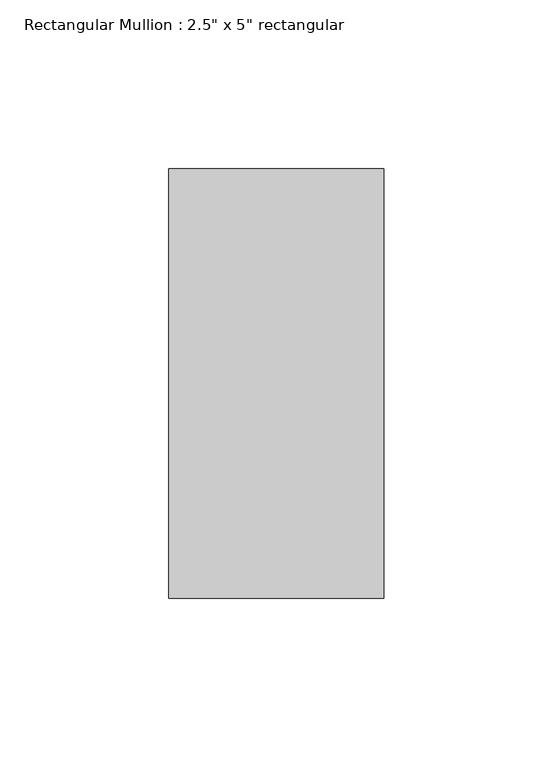
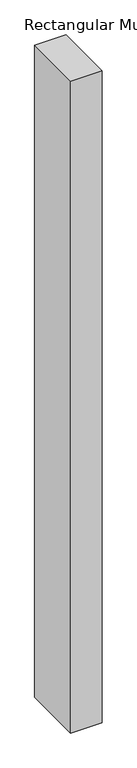
"""IFC4 building model written with IfcOpenShell, lengths in millimetres: member geometry."""

from ifc_helpers import new_model, si_unit, frame, origin, place, context, project, spatial, polyline, outline, extrude, source, transform, mapped, element, save


def member_3093b26a(model_context):
    return source(origin(), model_context, "Body", "SweptSolid", [
        extrude(outline(polyline([(31.75, 63.5), (31.75, -63.5), (-31.75, -63.5), (-31.75, 63.5), (31.75, 63.5)])), frame((0.0, 0.0, -1403.3499998), z_axis=(0.0, 0.0, 1.0), x_axis=(1.0, 0.0, 0.0)), (0.0, 0.0, 1.0), 1403.3499998),
    ])


if __name__ == "__main__":
    model = new_model("IFC4")
    model_context = context("Model", 3, world=origin())
    ifc_project = project(units=[si_unit("LENGTHUNIT", "METRE", prefix="MILLI")], contexts=[model_context])
    site = spatial("IfcSite", under=ifc_project)
    building = spatial("IfcBuilding", under=site)
    placement = place(None, origin())
    member_shape = member_3093b26a(model_context)
    element("IfcMember", 1, ObjectType="Rectangular Mullion : 2.5\" x 5\" rectangular", at=placement, inside=building, context=model_context, shape_type="MappedRepresentation", body=[
        mapped(member_shape, transform((0.0, 0.0, 0.0), x_axis=(1.0, 0.0, 0.0), y_axis=(0.0, 1.0, 0.0), z_axis=(0.0, 0.0, 1.0))),
    ])
    save(model, "model.ifc")

# Revit data of these elements
# Type "Rectangular Mullion : 2.5\" x 5\" rectangular"
#   built-in parameter 1007304 = 0.416667 (stored number, unit not read)
#   built-in parameter 1007301 = 0.104167 (stored number, unit not read)
#   built-in parameter 1007300 = 0.104167 (stored number, unit not read)
# Element 1 (IfcMember, "Rectangular Mullion : 2.5\" x 5\" rectangular")
#   Materials on its faces: "metal black"
# Materials
#   "metal black": class "Generic", colour RGB 120 120 120, transparency 0, Cost = 0
